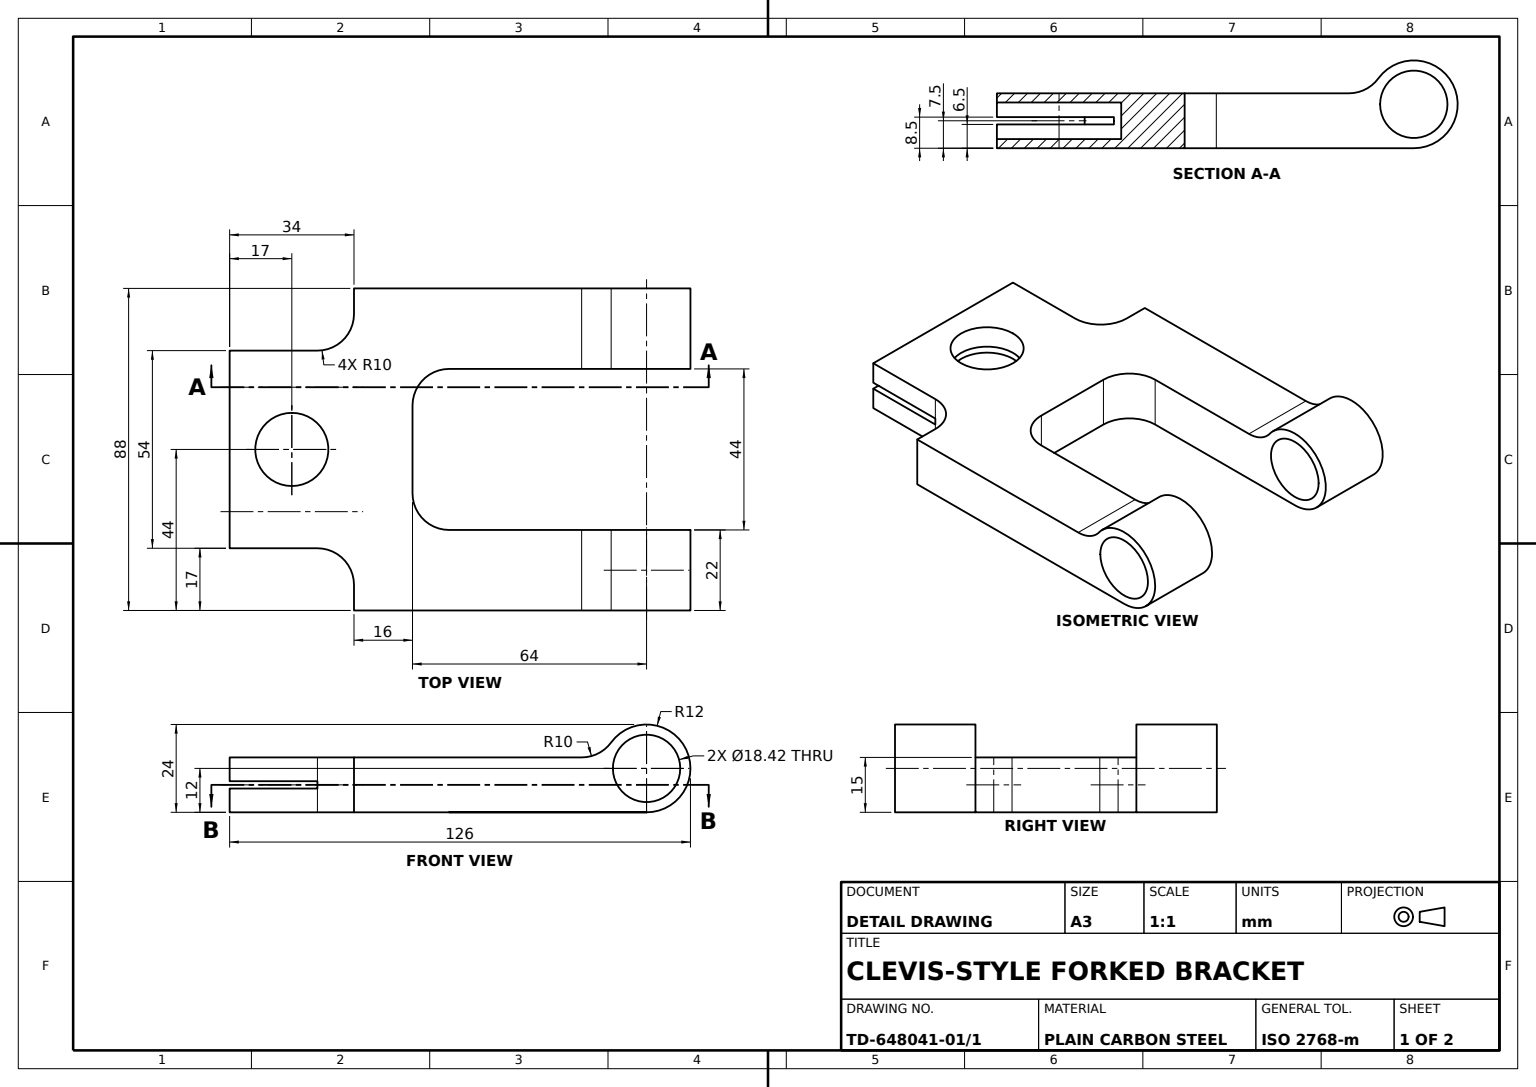
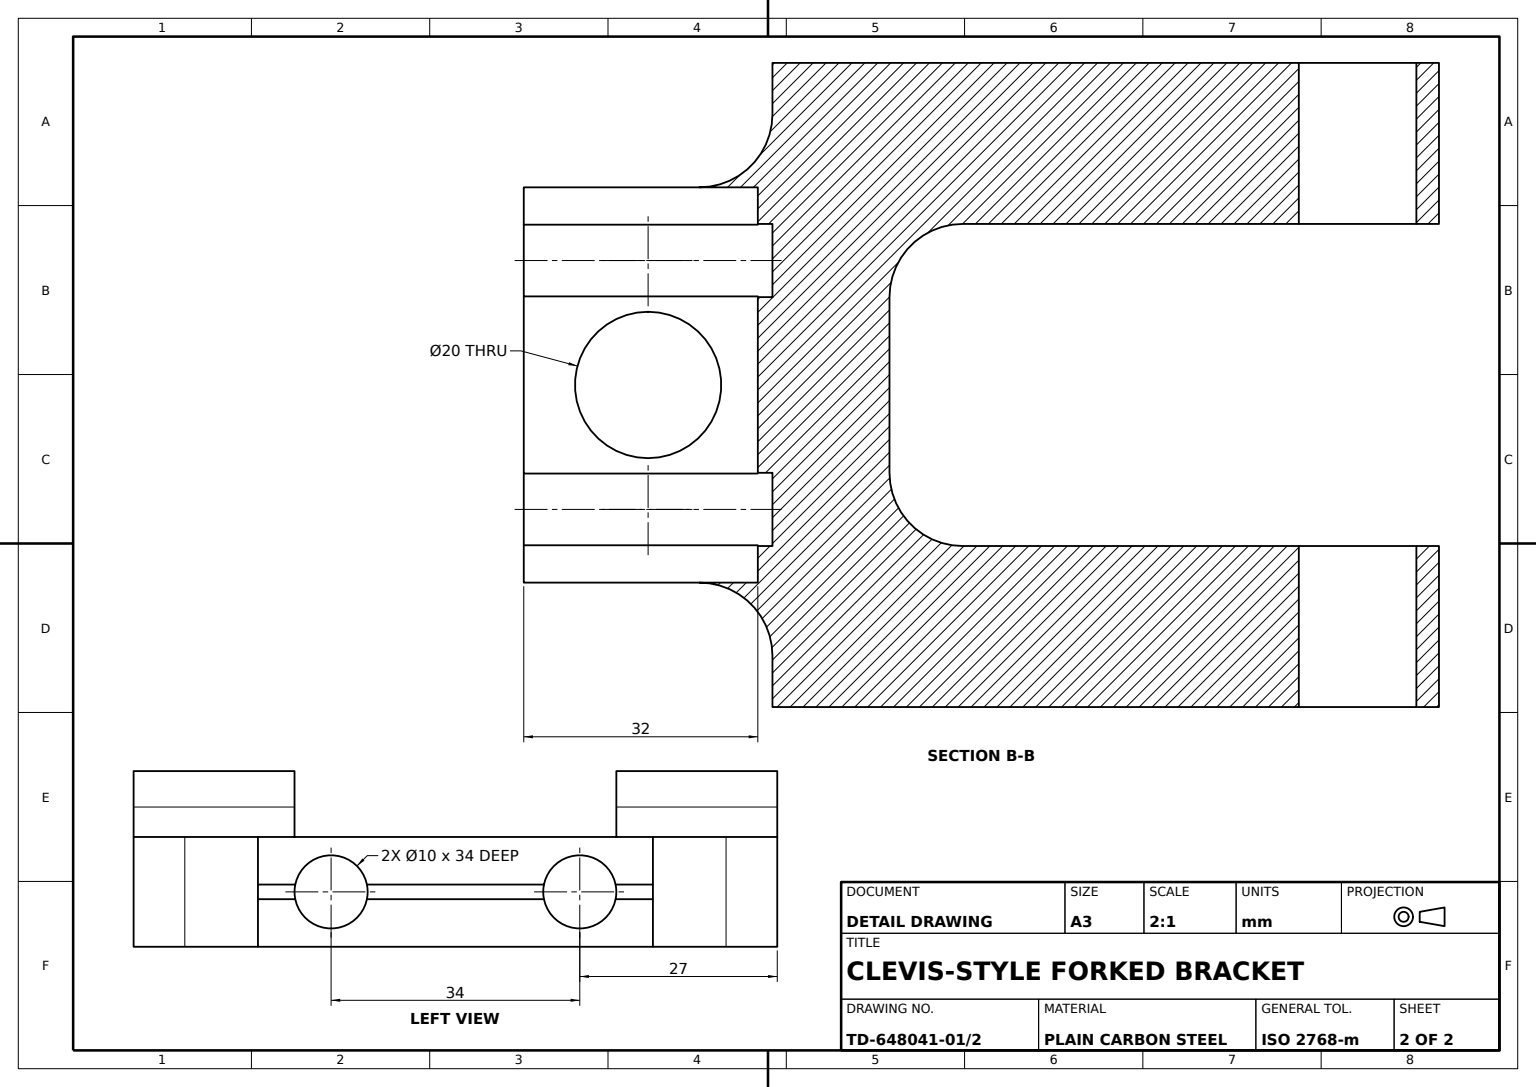
SolidWorks part; units mm, degrees
material "Plain Carbon Steel"
ref_plane "Front Plane" through (0, 0, 0) normal (0, 0, 1) x (1, 0, 0)
ref_plane "Top Plane" through (0, 0, 0) normal (0, 1, 0) x (1, 0, 0)
ref_plane "Right Plane" through (0, 0, 0) normal (1, 0, 0) x (0, 0, -1)
sketch "Base Plate Sketch" plane through (0, 0, 0) normal (0, 1, 0) x (1, 0, 0)
  line L0 (0, 44) -> (0, 22)
  line L1 (0, -44) -> (-64, -44)
  line L2 (0, 44) -> (-64, 44)
  line L4 (0, 22) -> (-54, 22)
  line L5 (0, -22) -> (-54, -22)
  line L7 (0, -22) -> (0, -44)
  line L8 (-64, -12) -> (-64, 12)
  line L9 (-114, 27) -> (-114, -27)
  line L10 (-114, -27) -> (-90, -27)
  line L11 (-80, -37) -> (-80, -44)
  line L12 (-80, -44) -> (-64, -44)
  line L13 (-80, 44) -> (-64, 44)
  line L14 (-80, 37) -> (-80, 44)
  line L15 (-114, 27) -> (-90, 27)
  line L16 (0, 22) -> (-64, 22) construction
  line L17 (0, -22) -> (-64, -22) construction
  arc A0 (-80, -37) -> (-90, -27) centre (-90, -37) ccw
  arc A1 (-80, 37) -> (-90, 27) centre (-90, 37) cw
  arc A2 (-54, 22) -> (-64, 12) centre (-54, 12) ccw
  arc A3 (-54, -22) -> (-64, -12) centre (-54, -12) cw
  circle A4 centre (-97, 0) radius 10
  point P4 (0, 0)
  point P16 (-114, 0)
  point P20 (-80, -27)
  dimension "D8" = 10
  dimension "D5" = 10
  dimension "D10" = 20
  dimension "D1" = 64
  dimension "D4" = 44
  dimension "D6" = 54
  dimension "D7" = 34
  dimension "D9" = 17
  dimension "D11" = 54
  dimension "D12" = 16
  dimension "D2" = 22
  dimension "D3" = 22
extrude "Base Plate" add sketch "Base Plate Sketch" along normal mid plane 15
sketch "Knuckle A Sketch" plane through (0, 0, 44) normal (0, 0, 1) x (1, 0, 0)
  circle A0 centre (0, 4.5) radius 12
  circle A1 centre (0, 4.5) radius 9
  dimension "D2" = 24
  dimension "D3" = 18
  dimension "D1" = 4.5
extrude "Knuckle A" add sketch "Knuckle A Sketch" against normal blind 22
sketch "Knuckle A Bore Sketch" plane through (0, 0, 44) normal (0, 0, 1) x (1, 0, 0)
  circle A0 centre (0, 4.5) radius 9.2108
  dimension "D1" = 18.4215
extrude "Knuckle A Bore" cut sketch "Knuckle A Bore Sketch" against normal blind 22
fillet "Knuckle A Blend R10" radius 10 1 edges at (-11.619, 7.5, 33)
sketch "Knuckle B Sketch" plane through (0, 0, -44) normal (0, 0, -1) x (-1, 0, 0)
  circle A0 centre (0, 4.5) radius 9.2108
  circle A1 centre (0, 4.5) radius 12
  dimension "D1" = 18.4215
  dimension "D2" = 24
extrude "Knuckle B" add sketch "Knuckle B Sketch" against normal blind 22
sketch "Knuckle B Bore Sketch" plane through (0, 0, -44) normal (0, 0, -1) x (-1, 0, 0)
  circle A0 centre (0, 4.5) radius 9.2108
  dimension "D1" = 18.4215
extrude "Knuckle B Bore" cut sketch "Knuckle B Bore Sketch" against normal blind 22
fillet "Knuckle B Blend R10" radius 10 1 edges at (-11.619, 7.5, -33)
sketch "Groove Cut Sketch" plane through (-114, 0, 0) normal (-1, 0, 0) x (0, 0, 1)
  line L0 (-27, -7.5) -> (27, -7.5) construction
  line L3 (-27, -1) -> (27, -1)
  line L4 (-27, 1) -> (27, 1)
  line L5 (27, 7.5) -> (27, -7.5) construction
  line L6 (-27, 7.5) -> (-27, -7.5) construction
  line L7 (27, 1) -> (27, -1)
  line L8 (-27, 1) -> (-27, -1)
  point P0 (-27, 0)
  point P1 (37, 0)
  point P7 (37, -1)
  point P9 (37, 1)
  dimension "D1" = 6.5
  dimension "D2" = 8.5
extrude "Groove Cut" cut sketch "Groove Cut Sketch" against normal blind 32
sketch "Hole Cut Sketch" plane through (-114, 0, 0) normal (-1, 0, 0) x (0, 0, 1)
  line L0 (-27, -1) -> (27, -1) construction
  line L1 (-27, -1) -> (-27, 1) construction
  circle A0 centre (-17, 0) radius 5
  circle A2 centre (17, 0) radius 5
  dimension "D1" = 10
  dimension "D4" = 10
  dimension "D2" = 10
  dimension "D3" = 10
  dimension "D5" = 1
extrude "Hole Cut" cut sketch "Hole Cut Sketch" against normal blind 34
